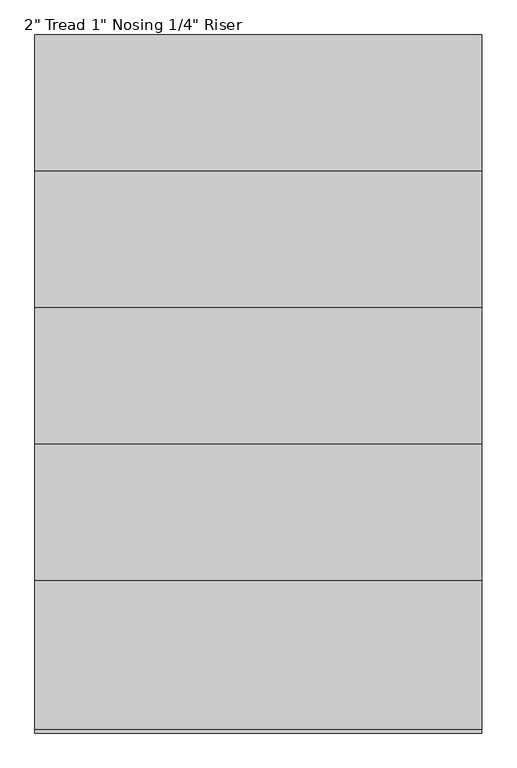
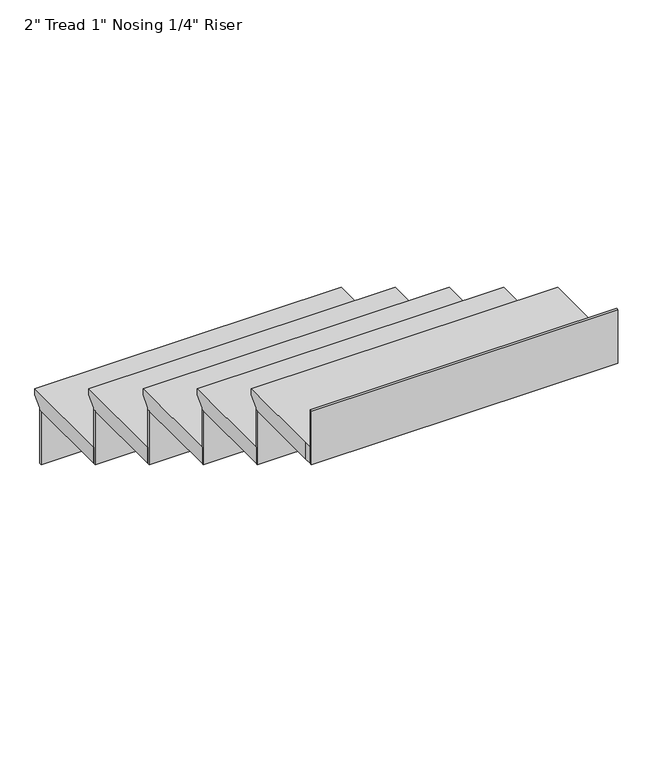
"""IFC4 building model written with IfcOpenShell, lengths in millimetres: stair flight geometry."""

from ifc_helpers import new_model, si_unit, origin, place, context, project, spatial, faceted_brep, source, transform, mapped, element, save


def stair_flight_788f3b80(model_context):
    return source(origin(), model_context, "Body", "Brep", [
        faceted_brep([(-803.1608498, 3514.5115866, 1335.6166667), (-803.1608498, 3514.5115866, 1354.6666667), (111.2391502, 3514.5115866, 1354.6666667), (111.2391502, 3514.5115866, 1335.6166667), (-803.1608498, 3489.1115866, 1310.2166667), (111.2391502, 3489.1115866, 1310.2166667), (-803.1608498, 3209.7115866, 1354.6666667), (111.2391502, 3209.7115866, 1354.6666667), (111.2391502, 3489.1115866, 1303.8666667), (111.2391502, 3209.7115866, 1303.8666667), (-803.1608498, 3209.7115866, 1303.8666667), (-803.1608498, 3489.1115866, 1303.8666667)], [[[0, 1, 2, 3]], [[4, 0, 3, 5]], [[2, 1, 6, 7]], [[8, 9, 10, 11]], [[2, 7, 9, 8, 5, 3]], [[8, 11, 4, 5]], [[6, 1, 0, 4, 11, 10]], [[7, 6, 10, 9]]]),
        faceted_brep([(-803.1608498, 3489.1115866, 1303.8666667), (-803.1608498, 3489.1115866, 1134.5333333), (-803.1608498, 3482.7615866, 1134.5333333), (-803.1608498, 3482.7615866, 1303.8666667), (111.2391502, 3489.1115866, 1303.8666667), (111.2391502, 3482.7615866, 1303.8666667), (111.2391502, 3482.7615866, 1134.5333333), (111.2391502, 3489.1115866, 1134.5333333)], [[[0, 1, 2, 3]], [[4, 5, 6, 7]], [[1, 0, 4, 7]], [[2, 1, 7, 6]], [[3, 2, 6, 5]], [[0, 3, 5, 4]]]),
        faceted_brep([(-803.1608498, 3209.7115866, 1473.2), (-803.1608498, 3209.7115866, 1303.8666667), (-803.1608498, 3203.3615866, 1303.8666667), (-803.1608498, 3203.3615866, 1473.2), (111.2391502, 3209.7115866, 1473.2), (111.2391502, 3203.3615866, 1473.2), (111.2391502, 3203.3615866, 1303.8666667), (111.2391502, 3209.7115866, 1303.8666667)], [[[0, 1, 2, 3]], [[4, 5, 6, 7]], [[1, 0, 4, 7]], [[2, 1, 7, 6]], [[3, 2, 6, 5]], [[0, 3, 5, 4]]]),
        faceted_brep([(111.2391502, 3235.1115866, 1524.0), (-803.1608498, 3235.1115866, 1524.0), (-803.1608498, 2930.3115866, 1524.0), (111.2391502, 2930.3115866, 1524.0), (111.2391502, 3209.7115866, 1473.2), (111.2391502, 2930.3115866, 1473.2), (-803.1608498, 2930.3115866, 1473.2), (-803.1608498, 3209.7115866, 1473.2), (111.2391502, 3209.7115866, 1479.55), (111.2391502, 3235.1115866, 1504.95), (-803.1608498, 3209.7115866, 1479.55), (-803.1608498, 3235.1115866, 1504.95)], [[[0, 1, 2, 3]], [[4, 5, 6, 7]], [[0, 3, 5, 4, 8, 9]], [[4, 7, 10, 8]], [[2, 1, 11, 10, 7, 6]], [[3, 2, 6, 5]], [[11, 1, 0, 9]], [[10, 11, 9, 8]]]),
        faceted_brep([(-803.1608498, 2930.3115866, 1642.5333333), (-803.1608498, 2930.3115866, 1473.2), (-803.1608498, 2923.9615866, 1473.2), (-803.1608498, 2923.9615866, 1642.5333333), (111.2391502, 2930.3115866, 1642.5333333), (111.2391502, 2923.9615866, 1642.5333333), (111.2391502, 2923.9615866, 1473.2), (111.2391502, 2930.3115866, 1473.2)], [[[0, 1, 2, 3]], [[4, 5, 6, 7]], [[1, 0, 4, 7]], [[2, 1, 7, 6]], [[3, 2, 6, 5]], [[0, 3, 5, 4]]]),
        faceted_brep([(111.2391502, 2955.7115866, 1693.3333333), (-803.1608498, 2955.7115866, 1693.3333333), (-803.1608498, 2650.9115866, 1693.3333333), (111.2391502, 2650.9115866, 1693.3333333), (111.2391502, 2930.3115866, 1642.5333333), (111.2391502, 2650.9115866, 1642.5333333), (-803.1608498, 2650.9115866, 1642.5333333), (-803.1608498, 2930.3115866, 1642.5333333), (111.2391502, 2930.3115866, 1648.8833333), (111.2391502, 2955.7115866, 1674.2833333), (-803.1608498, 2930.3115866, 1648.8833333), (-803.1608498, 2955.7115866, 1674.2833333)], [[[0, 1, 2, 3]], [[4, 5, 6, 7]], [[0, 3, 5, 4, 8, 9]], [[4, 7, 10, 8]], [[2, 1, 11, 10, 7, 6]], [[3, 2, 6, 5]], [[11, 1, 0, 9]], [[10, 11, 9, 8]]]),
        faceted_brep([(-803.1608498, 2650.9115866, 1811.8666667), (-803.1608498, 2650.9115866, 1642.5333333), (-803.1608498, 2644.5615866, 1642.5333333), (-803.1608498, 2644.5615866, 1811.8666667), (111.2391502, 2650.9115866, 1811.8666667), (111.2391502, 2644.5615866, 1811.8666667), (111.2391502, 2644.5615866, 1642.5333333), (111.2391502, 2650.9115866, 1642.5333333)], [[[0, 1, 2, 3]], [[4, 5, 6, 7]], [[1, 0, 4, 7]], [[2, 1, 7, 6]], [[3, 2, 6, 5]], [[0, 3, 5, 4]]]),
        faceted_brep([(111.2391502, 2676.3115866, 1862.6666667), (-803.1608498, 2676.3115866, 1862.6666667), (-803.1608498, 2371.5115866, 1862.6666667), (111.2391502, 2371.5115866, 1862.6666667), (111.2391502, 2650.9115866, 1811.8666667), (111.2391502, 2371.5115866, 1811.8666667), (-803.1608498, 2371.5115866, 1811.8666667), (-803.1608498, 2650.9115866, 1811.8666667), (111.2391502, 2650.9115866, 1818.2166667), (111.2391502, 2676.3115866, 1843.6166667), (-803.1608498, 2650.9115866, 1818.2166667), (-803.1608498, 2676.3115866, 1843.6166667)], [[[0, 1, 2, 3]], [[4, 5, 6, 7]], [[0, 3, 5, 4, 8, 9]], [[4, 7, 10, 8]], [[2, 1, 11, 10, 7, 6]], [[3, 2, 6, 5]], [[11, 1, 0, 9]], [[10, 11, 9, 8]]]),
        faceted_brep([(-803.1608498, 2092.1115866, 2150.5333333), (-803.1608498, 2092.1115866, 1981.2), (-803.1608498, 2085.7615866, 1981.2), (-803.1608498, 2085.7615866, 2150.5333333), (111.2391502, 2092.1115866, 2150.5333333), (111.2391502, 2085.7615866, 2150.5333333), (111.2391502, 2085.7615866, 1981.2), (111.2391502, 2092.1115866, 1981.2)], [[[0, 1, 2, 3]], [[4, 5, 6, 7]], [[1, 0, 4, 7]], [[2, 1, 7, 6]], [[3, 2, 6, 5]], [[0, 3, 5, 4]]]),
        faceted_brep([(-803.1608498, 2371.5115866, 1981.2), (-803.1608498, 2371.5115866, 1811.8666667), (-803.1608498, 2365.1615866, 1811.8666667), (-803.1608498, 2365.1615866, 1981.2), (111.2391502, 2371.5115866, 1981.2), (111.2391502, 2365.1615866, 1981.2), (111.2391502, 2365.1615866, 1811.8666667), (111.2391502, 2371.5115866, 1811.8666667)], [[[0, 1, 2, 3]], [[4, 5, 6, 7]], [[1, 0, 4, 7]], [[2, 1, 7, 6]], [[3, 2, 6, 5]], [[0, 3, 5, 4]]]),
        faceted_brep([(111.2391502, 2092.1115866, 2032.0), (111.2391502, 2117.5115866, 2032.0), (111.2391502, 2396.9115866, 2032.0), (-803.1608498, 2396.9115866, 2032.0), (-803.1608498, 2117.5115866, 2032.0), (-803.1608498, 2092.1115866, 2032.0), (111.2391502, 2117.5115866, 1981.2), (111.2391502, 2092.1115866, 1981.2), (-803.1608498, 2092.1115866, 1981.2), (-803.1608498, 2117.5115866, 1981.2), (-803.1608498, 2371.5115866, 1981.2), (111.2391502, 2371.5115866, 1981.2), (111.2391502, 2371.5115866, 1987.55), (111.2391502, 2396.9115866, 2012.95), (-803.1608498, 2371.5115866, 1987.55), (-803.1608498, 2396.9115866, 2012.95)], [[[0, 1, 2, 3, 4, 5]], [[6, 7, 8, 9, 10, 11]], [[1, 0, 7, 6]], [[2, 1, 6, 11, 12, 13]], [[11, 10, 14, 12]], [[4, 3, 15, 14, 10, 9]], [[5, 4, 9, 8]], [[0, 5, 8, 7]], [[15, 3, 2, 13]], [[14, 15, 13, 12]]]),
    ])


if __name__ == "__main__":
    model = new_model("IFC4")
    model_context = context("Model", 3, world=origin())
    ifc_project = project(units=[si_unit("LENGTHUNIT", "METRE", prefix="MILLI")], contexts=[model_context])
    site = spatial("IfcSite", under=ifc_project)
    building = spatial("IfcBuilding", under=site)
    placement = place(None, origin())
    stair_flight_shape = stair_flight_788f3b80(model_context)
    element("IfcStairFlight", 1, ObjectType="2\" Tread 1\" Nosing 1/4\" Riser", at=placement, inside=building, context=model_context, shape_type="MappedRepresentation", body=[
        mapped(stair_flight_shape, transform((0.0, 0.0, 0.0), x_axis=(1.0, 0.0, 0.0), y_axis=(0.0, 1.0, 0.0), z_axis=(0.0, 0.0, 1.0))),
    ])
    save(model, "model.ifc")
